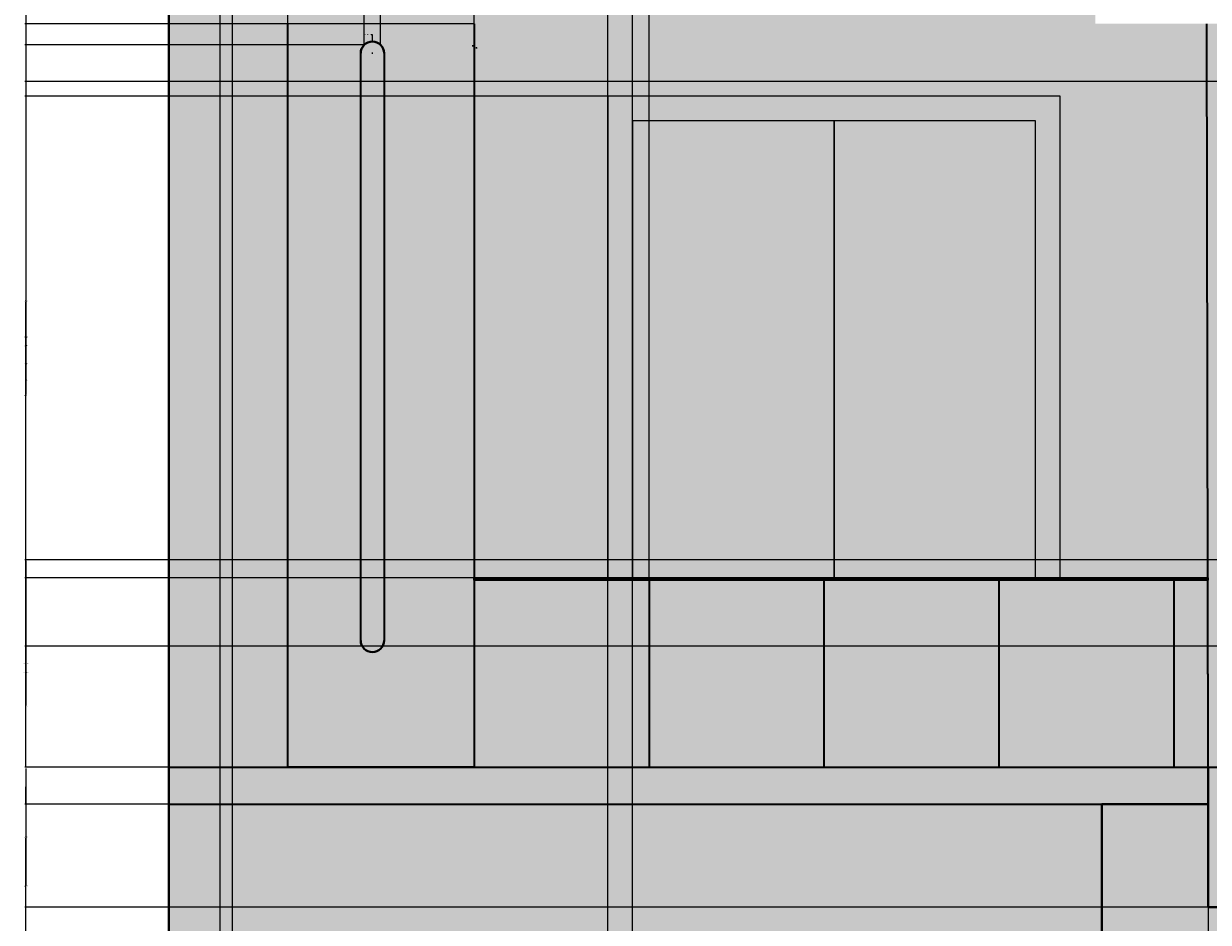
# Model space of a CAD drawing. Units: feet. Extents: x 2368 to 2738, y 1285 to 1782.
# Tile 2 of 6: x 2368 to 2561, y 1464 to 1610. Entities that reach past the tile are written whole.
import ezdxf

# ---------------------------------------------------------------- set-up
doc = ezdxf.new("R2010")
doc.units = ezdxf.units.FT
for name, color, linetype, lineweight in [('A-ANNO-DIMS', 2, 'Continuous', 18), ('A-DOOR', 3, 'Continuous', 25), ('A-ELEV', 7, 'Continuous', 35), ('A-ELEV-PATT', 252, 'Continuous', 13)]:
    doc.layers.add(name, color=color, linetype=linetype, lineweight=lineweight)
doc.styles.get("Standard").update_dxf_attribs({"font": 'arial.ttf'})
doc.dimstyles.get("Standard").update_dxf_attribs({"dimtxt": 0.18, "dimasz": 0.18, "dimexe": 0.18, "dimexo": 0.0625, "dimgap": 0.09, "dimtad": 0, "dimtih": 1, "dimtoh": 1, "dimdec": 1, "dimzin": 0, "dimdsep": 46, "dimlunit": 3, "dimtxsty": 'Standard', "dimcen": 0.09, "dimadec": 0, "dimazin": 0, "dimtfac": 1, "dimtdec": 1, "dimtofl": 0, "dimtmove": 0, "dimatfit": 3, "dimfxl": 1, "dimtolj": 1, "dimtzin": 0, "dimarcsym": 0})

# ---------------------------------------------------------------- blocks, each defined once
blk = doc.blocks.new('*D6')
at = {"layer": 'A-ANNO-DIMS', "color": 0, "lineweight": -2, "transparency": 16777216}
for p, q in [((2391.48, 1482.86), (2368.11, 1482.86)), ((2368.29, 1482.68), (2368.29, 1469.65)), ((2368.29, 1456.26), (2368.29, 1469.29)), ((2399.84, 1456.08), (2368.11, 1456.08))]:
    blk.add_line(p, q, dxfattribs=at)
at = {"layer": 'A-ANNO-DIMS', "color": 0, "transparency": 16777216}
for points in [[(2368.26, 1482.68), (2368.32, 1482.68), (2368.29, 1482.86)], [(2368.26, 1456.26), (2368.32, 1456.26), (2368.29, 1456.08)]]:
    blk.add_solid(points, dxfattribs=at)
at = {"layer": 'Defpoints', "color": 0, "transparency": 16777216}
for p in [(2368.29, 1482.86), (2391.54, 1482.86), (2399.91, 1456.08)]:
    blk.add_point(p, dxfattribs=at)
at = {"layer": 'A-ANNO-DIMS', "color": 0, "transparency": 16777216, "insert": (2368.29, 1469.47), "char_height": 0.18, "attachment_point": 5}
blk.add_mtext('\\A1;26.77', dxfattribs=at)
blk = doc.blocks.new('*D7')
at = {"layer": 'A-ANNO-DIMS', "color": 0, "lineweight": -2, "transparency": 16777216}
for p, q in [((2391.48, 1488.86), (2368.11, 1488.86)), ((2368.29, 1488.68), (2368.29, 1486.04)), ((2368.29, 1483.04), (2368.29, 1485.67)), ((2391.48, 1482.86), (2368.11, 1482.86))]:
    blk.add_line(p, q, dxfattribs=at)
at = {"layer": 'A-ANNO-DIMS', "color": 0, "transparency": 16777216}
for points in [[(2368.26, 1488.68), (2368.32, 1488.68), (2368.29, 1488.86)], [(2368.26, 1483.04), (2368.32, 1483.04), (2368.29, 1482.86)]]:
    blk.add_solid(points, dxfattribs=at)
at = {"layer": 'Defpoints', "color": 0, "transparency": 16777216}
for p in [(2368.29, 1488.86), (2391.54, 1488.86), (2391.54, 1482.86)]:
    blk.add_point(p, dxfattribs=at)
at = {"layer": 'A-ANNO-DIMS', "color": 0, "transparency": 16777216, "insert": (2368.29, 1485.86), "char_height": 0.18, "attachment_point": 5}
blk.add_mtext('\\A1;6', dxfattribs=at)
blk = doc.blocks.new('*D8')
at = {"layer": 'A-ANNO-DIMS', "color": 0, "lineweight": -2, "transparency": 16777216}
for p, q in [((2391.48, 1614.86), (2368.11, 1614.86)), ((2368.29, 1614.68), (2368.29, 1552.04)), ((2368.29, 1489.04), (2368.29, 1551.67)), ((2391.48, 1488.86), (2368.11, 1488.86))]:
    blk.add_line(p, q, dxfattribs=at)
at = {"layer": 'A-ANNO-DIMS', "color": 0, "transparency": 16777216}
for points in [[(2368.26, 1614.68), (2368.32, 1614.68), (2368.29, 1614.86)], [(2368.26, 1489.04), (2368.32, 1489.04), (2368.29, 1488.86)]]:
    blk.add_solid(points, dxfattribs=at)
at = {"layer": 'Defpoints', "color": 0, "transparency": 16777216}
for p in [(2368.29, 1614.86), (2391.54, 1614.86), (2391.54, 1488.86)]:
    blk.add_point(p, dxfattribs=at)
at = {"layer": 'A-ANNO-DIMS', "color": 0, "transparency": 16777216, "insert": (2368.29, 1551.86), "char_height": 0.18, "attachment_point": 5}
blk.add_mtext('\\A1;126', dxfattribs=at)
blk = doc.blocks.new('*D19')
at = {"layer": 'A-ANNO-DIMS', "color": 0, "lineweight": -2, "transparency": 16777216}
for p, q in [((2560.8, 1466.04), (2560.8, 1285.43)), ((2543.45, 1350.79), (2543.45, 1285.43)), ((2543.63, 1285.61), (2551.74, 1285.61)), ((2560.62, 1285.61), (2552.51, 1285.61))]:
    blk.add_line(p, q, dxfattribs=at)
at = {"layer": 'A-ANNO-DIMS', "color": 0, "transparency": 16777216}
for points in [[(2543.63, 1285.64), (2543.63, 1285.58), (2543.45, 1285.61)], [(2560.62, 1285.64), (2560.62, 1285.58), (2560.8, 1285.61)]]:
    blk.add_solid(points, dxfattribs=at)
at = {"layer": 'Defpoints', "color": 0, "transparency": 16777216}
for p in [(2560.8, 1466.1), (2543.45, 1350.86), (2560.8, 1285.61)]:
    blk.add_point(p, dxfattribs=at)
at = {"layer": 'A-ANNO-DIMS', "color": 0, "transparency": 16777216, "insert": (2552.12, 1285.61), "char_height": 0.18, "attachment_point": 5}
blk.add_mtext('\\A1;17.35', dxfattribs=at)
blk = doc.blocks.new('*D24')
at = {"layer": 'A-ANNO-DIMS', "color": 0, "lineweight": -2, "transparency": 16777216}
for p, q in [((2399.91, 1456.15), (2399.91, 1782.11)), ((2400.09, 1781.93), (2400.76, 1781.93)), ((2401.73, 1781.93), (2401.06, 1781.93)), ((2401.91, 1454.15), (2401.91, 1782.11))]:
    blk.add_line(p, q, dxfattribs=at)
at = {"layer": 'A-ANNO-DIMS', "color": 0, "transparency": 16777216}
for points in [[(2400.09, 1781.96), (2400.09, 1781.9), (2399.91, 1781.93)], [(2401.73, 1781.96), (2401.73, 1781.9), (2401.91, 1781.93)]]:
    blk.add_solid(points, dxfattribs=at)
at = {"layer": 'Defpoints', "color": 0, "transparency": 16777216}
for p in [(2401.91, 1781.93), (2399.91, 1456.08), (2401.91, 1454.08)]:
    blk.add_point(p, dxfattribs=at)
at = {"layer": 'A-ANNO-DIMS', "color": 0, "transparency": 16777216, "insert": (2400.91, 1781.93), "char_height": 0.18, "attachment_point": 5}
blk.add_mtext('\\A1;2', dxfattribs=at)
blk = doc.blocks.new('*D30')
at = {"layer": 'A-ANNO-DIMS', "color": 0, "lineweight": -2, "transparency": 16777216}
for p, q in [((2463.03, 1460.16), (2463.03, 1782.11)), ((2463.21, 1781.93), (2464.88, 1781.93)), ((2466.85, 1781.93), (2465.18, 1781.93)), ((2467.03, 1456.16), (2467.03, 1782.11))]:
    blk.add_line(p, q, dxfattribs=at)
at = {"layer": 'A-ANNO-DIMS', "color": 0, "transparency": 16777216}
for points in [[(2463.21, 1781.96), (2463.21, 1781.9), (2463.03, 1781.93)], [(2466.85, 1781.96), (2466.85, 1781.9), (2467.03, 1781.93)]]:
    blk.add_solid(points, dxfattribs=at)
at = {"layer": 'Defpoints', "color": 0, "transparency": 16777216}
for p in [(2467.03, 1781.93), (2463.03, 1460.1), (2467.03, 1456.1)]:
    blk.add_point(p, dxfattribs=at)
at = {"layer": 'A-ANNO-DIMS', "color": 0, "transparency": 16777216, "insert": (2465.03, 1781.93), "char_height": 0.18, "attachment_point": 5}
blk.add_mtext('\\A1;4', dxfattribs=at)
blk = doc.blocks.new('*D36')
at = {"layer": 'A-ANNO-DIMS', "color": 0, "lineweight": -2, "transparency": 16777216}
for p, q in [((2701.6, 1488.86), (2368.11, 1488.86)), ((2368.29, 1488.68), (2368.29, 1477.66)), ((2368.29, 1466.28), (2368.29, 1477.3)), ((2701.6, 1466.1), (2368.11, 1466.1))]:
    blk.add_line(p, q, dxfattribs=at)
at = {"layer": 'A-ANNO-DIMS', "color": 0, "transparency": 16777216}
for points in [[(2368.26, 1488.68), (2368.32, 1488.68), (2368.29, 1488.86)], [(2368.26, 1466.28), (2368.32, 1466.28), (2368.29, 1466.1)]]:
    blk.add_solid(points, dxfattribs=at)
at = {"layer": 'Defpoints', "color": 0, "transparency": 16777216}
for p in [(2368.29, 1488.86), (2701.66, 1488.86), (2701.66, 1466.1)]:
    blk.add_point(p, dxfattribs=at)
at = {"layer": 'A-ANNO-DIMS', "color": 0, "transparency": 16777216, "insert": (2368.29, 1477.48), "char_height": 0.18, "attachment_point": 5}
blk.add_mtext('\\A1;22.754', dxfattribs=at)
blk = doc.blocks.new('*D37')
at = {"layer": 'A-ANNO-DIMS', "color": 0, "lineweight": -2, "transparency": 16777216}
for p, q in [((2701.6, 1522.63), (2368.11, 1522.63)), ((2368.29, 1522.45), (2368.29, 1505.93)), ((2368.29, 1489.04), (2368.29, 1505.56)), ((2701.6, 1488.86), (2368.11, 1488.86))]:
    blk.add_line(p, q, dxfattribs=at)
at = {"layer": 'A-ANNO-DIMS', "color": 0, "transparency": 16777216}
for points in [[(2368.26, 1522.45), (2368.32, 1522.45), (2368.29, 1522.63)], [(2368.26, 1489.04), (2368.32, 1489.04), (2368.29, 1488.86)]]:
    blk.add_solid(points, dxfattribs=at)
at = {"layer": 'Defpoints', "color": 0, "transparency": 16777216}
for p in [(2368.29, 1522.63), (2701.66, 1522.63), (2701.66, 1488.86)]:
    blk.add_point(p, dxfattribs=at)
at = {"layer": 'A-ANNO-DIMS', "color": 0, "transparency": 16777216, "insert": (2368.29, 1505.74), "char_height": 0.18, "attachment_point": 5}
blk.add_mtext('\\A1;33.776', dxfattribs=at)
blk = doc.blocks.new('*D41')
at = {"layer": 'A-ANNO-DIMS', "color": 0, "lineweight": -2, "transparency": 16777216}
for p, q in [((2391.54, 1488.92), (2391.54, 1782.11)), ((2391.72, 1781.93), (2400.79, 1781.93)), ((2410.77, 1781.93), (2401.7, 1781.93)), ((2410.95, 1488.92), (2410.95, 1782.11))]:
    blk.add_line(p, q, dxfattribs=at)
at = {"layer": 'A-ANNO-DIMS', "color": 0, "transparency": 16777216}
for points in [[(2391.72, 1781.96), (2391.72, 1781.9), (2391.54, 1781.93)], [(2410.77, 1781.96), (2410.77, 1781.9), (2410.95, 1781.93)]]:
    blk.add_solid(points, dxfattribs=at)
at = {"layer": 'Defpoints', "color": 0, "transparency": 16777216}
for p in [(2410.95, 1781.93), (2391.54, 1488.86), (2410.95, 1488.86)]:
    blk.add_point(p, dxfattribs=at)
at = {"layer": 'A-ANNO-DIMS', "color": 0, "transparency": 16777216, "insert": (2401.24, 1781.93), "char_height": 0.18, "attachment_point": 5}
blk.add_mtext('\\A1;19.406', dxfattribs=at)
blk = doc.blocks.new('*D42')
at = {"layer": 'A-ANNO-DIMS', "color": 0, "lineweight": -2, "transparency": 16777216}
for p, q in [((2410.88, 1609.91), (2368.11, 1609.91)), ((2368.29, 1609.73), (2368.29, 1549.56)), ((2368.29, 1489.04), (2368.29, 1549.2)), ((2410.88, 1488.86), (2368.11, 1488.86))]:
    blk.add_line(p, q, dxfattribs=at)
at = {"layer": 'A-ANNO-DIMS', "color": 0, "transparency": 16777216}
for points in [[(2368.26, 1609.73), (2368.32, 1609.73), (2368.29, 1609.91)], [(2368.26, 1489.04), (2368.32, 1489.04), (2368.29, 1488.86)]]:
    blk.add_solid(points, dxfattribs=at)
at = {"layer": 'Defpoints', "color": 0, "transparency": 16777216}
for p in [(2368.29, 1609.91), (2410.95, 1609.91), (2410.95, 1488.86)]:
    blk.add_point(p, dxfattribs=at)
at = {"layer": 'A-ANNO-DIMS', "color": 0, "transparency": 16777216, "insert": (2368.29, 1549.38), "char_height": 0.18, "attachment_point": 5}
blk.add_mtext('\\A1;121.05', dxfattribs=at)
blk = doc.blocks.new('*D43')
at = {"layer": 'A-ANNO-DIMS', "color": 0, "lineweight": -2, "transparency": 16777216}
for p, q in [((2410.95, 1609.97), (2410.95, 1782.11)), ((2411.13, 1781.93), (2416.69, 1781.93)), ((2423.16, 1781.93), (2417.6, 1781.93)), ((2423.34, 1606.5), (2423.34, 1782.11))]:
    blk.add_line(p, q, dxfattribs=at)
at = {"layer": 'A-ANNO-DIMS', "color": 0, "transparency": 16777216}
for points in [[(2411.13, 1781.96), (2411.13, 1781.9), (2410.95, 1781.93)], [(2423.16, 1781.96), (2423.16, 1781.9), (2423.34, 1781.93)]]:
    blk.add_solid(points, dxfattribs=at)
at = {"layer": 'Defpoints', "color": 0, "transparency": 16777216}
for p in [(2423.34, 1781.93), (2410.95, 1609.91), (2423.34, 1606.44)]:
    blk.add_point(p, dxfattribs=at)
at = {"layer": 'A-ANNO-DIMS', "color": 0, "transparency": 16777216, "insert": (2417.15, 1781.93), "char_height": 0.18, "attachment_point": 5}
blk.add_mtext('\\A1;12.396', dxfattribs=at)
blk = doc.blocks.new('*D44')
at = {"layer": 'A-ANNO-DIMS', "color": 0, "lineweight": -2, "transparency": 16777216}
for p, q in [((2423.34, 1606.5), (2423.34, 1782.11)), ((2423.52, 1781.93), (2424.36, 1781.93)), ((2425.85, 1781.93), (2425.01, 1781.93)), ((2426.03, 1606.5), (2426.03, 1782.11))]:
    blk.add_line(p, q, dxfattribs=at)
at = {"layer": 'A-ANNO-DIMS', "color": 0, "transparency": 16777216}
for points in [[(2423.52, 1781.96), (2423.52, 1781.9), (2423.34, 1781.93)], [(2425.85, 1781.96), (2425.85, 1781.9), (2426.03, 1781.93)]]:
    blk.add_solid(points, dxfattribs=at)
at = {"layer": 'Defpoints', "color": 0, "transparency": 16777216}
for p in [(2426.03, 1781.93), (2423.34, 1606.44), (2426.03, 1606.44)]:
    blk.add_point(p, dxfattribs=at)
at = {"layer": 'A-ANNO-DIMS', "color": 0, "transparency": 16777216, "insert": (2424.69, 1781.93), "char_height": 0.18, "attachment_point": 5}
blk.add_mtext('\\A1;2.69', dxfattribs=at)
blk = doc.blocks.new('*D45')
at = {"layer": 'A-ANNO-DIMS', "color": 0, "lineweight": -2, "transparency": 16777216}
for p, q in [((2426.03, 1606.5), (2426.03, 1782.11)), ((2426.21, 1781.93), (2433.19, 1781.93)), ((2441.07, 1781.93), (2434.1, 1781.93)), ((2441.25, 1609.97), (2441.25, 1782.11))]:
    blk.add_line(p, q, dxfattribs=at)
at = {"layer": 'A-ANNO-DIMS', "color": 0, "transparency": 16777216}
for points in [[(2426.21, 1781.96), (2426.21, 1781.9), (2426.03, 1781.93)], [(2441.07, 1781.96), (2441.07, 1781.9), (2441.25, 1781.93)]]:
    blk.add_solid(points, dxfattribs=at)
at = {"layer": 'Defpoints', "color": 0, "transparency": 16777216}
for p in [(2441.25, 1781.93), (2441.25, 1609.91), (2426.03, 1606.44)]:
    blk.add_point(p, dxfattribs=at)
at = {"layer": 'A-ANNO-DIMS', "color": 0, "transparency": 16777216, "insert": (2433.64, 1781.93), "char_height": 0.18, "attachment_point": 5}
blk.add_mtext('\\A1;15.216', dxfattribs=at)
blk = doc.blocks.new('*D46')
at = {"layer": 'A-ANNO-DIMS', "color": 0, "lineweight": -2, "transparency": 16777216}
for p, q in [((2422.98, 1508.55), (2368.11, 1508.55)), ((2368.29, 1508.37), (2368.29, 1498.89)), ((2368.29, 1489.04), (2368.29, 1498.52)), ((2441.19, 1488.86), (2368.11, 1488.86))]:
    blk.add_line(p, q, dxfattribs=at)
at = {"layer": 'A-ANNO-DIMS', "color": 0, "transparency": 16777216}
for points in [[(2368.26, 1508.37), (2368.32, 1508.37), (2368.29, 1508.55)], [(2368.26, 1489.04), (2368.32, 1489.04), (2368.29, 1488.86)]]:
    blk.add_solid(points, dxfattribs=at)
at = {"layer": 'Defpoints', "color": 0, "transparency": 16777216}
for p in [(2368.29, 1508.55), (2423.04, 1508.55), (2441.25, 1488.86)]:
    blk.add_point(p, dxfattribs=at)
at = {"layer": 'A-ANNO-DIMS', "color": 0, "transparency": 16777216, "insert": (2368.29, 1498.7), "char_height": 0.18, "attachment_point": 5}
blk.add_mtext('\\A1;19.7', dxfattribs=at)
blk = doc.blocks.new('*D47')
at = {"layer": 'A-ANNO-DIMS', "color": 0, "lineweight": -2, "transparency": 16777216}
for p, q in [((2423.28, 1606.44), (2368.11, 1606.44)), ((2368.29, 1606.26), (2368.29, 1557.68)), ((2368.29, 1508.73), (2368.29, 1557.32)), ((2422.98, 1508.55), (2368.11, 1508.55))]:
    blk.add_line(p, q, dxfattribs=at)
at = {"layer": 'A-ANNO-DIMS', "color": 0, "transparency": 16777216}
for points in [[(2368.26, 1606.26), (2368.32, 1606.26), (2368.29, 1606.44)], [(2368.26, 1508.73), (2368.32, 1508.73), (2368.29, 1508.55)]]:
    blk.add_solid(points, dxfattribs=at)
at = {"layer": 'Defpoints', "color": 0, "transparency": 16777216}
for p in [(2368.29, 1606.44), (2423.34, 1606.44), (2423.04, 1508.55)]:
    blk.add_point(p, dxfattribs=at)
at = {"layer": 'A-ANNO-DIMS', "color": 0, "transparency": 16777216, "insert": (2368.29, 1557.5), "char_height": 0.18, "attachment_point": 5}
blk.add_mtext('\\A1;97.89', dxfattribs=at)
blk = doc.blocks.new('*D48')
at = {"layer": 'A-ANNO-DIMS', "color": 0, "lineweight": -2, "transparency": 16777216}
for p, q in [((2441.19, 1519.71), (2368.11, 1519.71)), ((2368.29, 1519.53), (2368.29, 1504.47)), ((2368.29, 1489.04), (2368.29, 1504.1)), ((2441.19, 1488.86), (2368.11, 1488.86))]:
    blk.add_line(p, q, dxfattribs=at)
at = {"layer": 'A-ANNO-DIMS', "color": 0, "transparency": 16777216}
for points in [[(2368.26, 1519.53), (2368.32, 1519.53), (2368.29, 1519.71)], [(2368.26, 1489.04), (2368.32, 1489.04), (2368.29, 1488.86)]]:
    blk.add_solid(points, dxfattribs=at)
at = {"layer": 'Defpoints', "color": 0, "transparency": 16777216}
for p in [(2368.29, 1519.71), (2441.25, 1519.71), (2441.25, 1488.86)]:
    blk.add_point(p, dxfattribs=at)
at = {"layer": 'A-ANNO-DIMS', "color": 0, "transparency": 16777216, "insert": (2368.29, 1504.28), "char_height": 0.18, "attachment_point": 5}
blk.add_mtext('\\A1;30.856', dxfattribs=at)
blk = doc.blocks.new('*D49')
at = {"layer": 'A-ANNO-DIMS', "color": 0, "lineweight": -2, "transparency": 16777216}
for p, q in [((2441.19, 1609.91), (2368.11, 1609.91)), ((2368.29, 1609.73), (2368.29, 1564.99)), ((2368.29, 1519.89), (2368.29, 1564.63)), ((2441.19, 1519.71), (2368.11, 1519.71))]:
    blk.add_line(p, q, dxfattribs=at)
at = {"layer": 'A-ANNO-DIMS', "color": 0, "transparency": 16777216}
for points in [[(2368.26, 1609.73), (2368.32, 1609.73), (2368.29, 1609.91)], [(2368.26, 1519.89), (2368.32, 1519.89), (2368.29, 1519.71)]]:
    blk.add_solid(points, dxfattribs=at)
at = {"layer": 'Defpoints', "color": 0, "transparency": 16777216}
for p in [(2368.29, 1609.91), (2441.25, 1609.91), (2441.25, 1519.71)]:
    blk.add_point(p, dxfattribs=at)
at = {"layer": 'A-ANNO-DIMS', "color": 0, "transparency": 16777216, "insert": (2368.29, 1564.81), "char_height": 0.18, "attachment_point": 5}
blk.add_mtext('\\A1;90.2', dxfattribs=at)
blk = doc.blocks.new('*D50')
at = {"layer": 'A-ANNO-DIMS', "color": 0, "lineweight": -2, "transparency": 16777216}
for p, q in [((2441.25, 1519.77), (2441.25, 1782.11)), ((2441.43, 1781.93), (2455.03, 1781.93)), ((2469.55, 1781.93), (2455.96, 1781.93)), ((2469.73, 1519.4), (2469.73, 1782.11))]:
    blk.add_line(p, q, dxfattribs=at)
at = {"layer": 'A-ANNO-DIMS', "color": 0, "transparency": 16777216}
for points in [[(2441.43, 1781.96), (2441.43, 1781.9), (2441.25, 1781.93)], [(2469.55, 1781.96), (2469.55, 1781.9), (2469.73, 1781.93)]]:
    blk.add_solid(points, dxfattribs=at)
at = {"layer": 'Defpoints', "color": 0, "transparency": 16777216}
for p in [(2469.73, 1781.93), (2441.25, 1519.71), (2469.73, 1519.33)]:
    blk.add_point(p, dxfattribs=at)
at = {"layer": 'A-ANNO-DIMS', "color": 0, "transparency": 16777216, "insert": (2455.49, 1781.93), "char_height": 0.18, "attachment_point": 5}
blk.add_mtext('\\A1;28.486', dxfattribs=at)
blk = doc.blocks.new('*D51')
at = {"layer": 'A-ANNO-DIMS', "color": 0, "lineweight": -2, "transparency": 16777216}
for p, q in [((2462.97, 1598.1), (2368.11, 1598.1)), ((2368.29, 1597.92), (2368.29, 1559.09)), ((2368.29, 1519.89), (2368.29, 1558.72)), ((2462.97, 1519.71), (2368.11, 1519.71))]:
    blk.add_line(p, q, dxfattribs=at)
at = {"layer": 'A-ANNO-DIMS', "color": 0, "transparency": 16777216}
for points in [[(2368.26, 1597.92), (2368.32, 1597.92), (2368.29, 1598.1)], [(2368.26, 1519.89), (2368.32, 1519.89), (2368.29, 1519.71)]]:
    blk.add_solid(points, dxfattribs=at)
at = {"layer": 'Defpoints', "color": 0, "transparency": 16777216}
for p in [(2368.29, 1598.1), (2463.03, 1598.1), (2463.03, 1519.71)]:
    blk.add_point(p, dxfattribs=at)
at = {"layer": 'A-ANNO-DIMS', "color": 0, "transparency": 16777216, "insert": (2368.29, 1558.9), "char_height": 0.18, "attachment_point": 5}
blk.add_mtext('\\A1;78.39', dxfattribs=at)
blk = doc.blocks.new('*D52')
at = {"layer": 'A-ANNO-DIMS', "color": 0, "lineweight": -2, "transparency": 16777216}
for p, q in [((2463.03, 1598.16), (2463.03, 1782.11)), ((2463.21, 1781.93), (2464.88, 1781.93)), ((2466.85, 1781.93), (2465.18, 1781.93)), ((2467.03, 1594.16), (2467.03, 1782.11))]:
    blk.add_line(p, q, dxfattribs=at)
at = {"layer": 'A-ANNO-DIMS', "color": 0, "transparency": 16777216}
for points in [[(2463.21, 1781.96), (2463.21, 1781.9), (2463.03, 1781.93)], [(2466.85, 1781.96), (2466.85, 1781.9), (2467.03, 1781.93)]]:
    blk.add_solid(points, dxfattribs=at)
at = {"layer": 'Defpoints', "color": 0, "transparency": 16777216}
for p in [(2467.03, 1781.93), (2463.03, 1598.1), (2467.03, 1594.1)]:
    blk.add_point(p, dxfattribs=at)
at = {"layer": 'A-ANNO-DIMS', "color": 0, "transparency": 16777216, "insert": (2465.03, 1781.93), "char_height": 0.18, "attachment_point": 5}
blk.add_mtext('\\A1;4', dxfattribs=at)
blk = doc.blocks.new('*D60')
at = {"layer": 'A-ANNO-DIMS', "color": 0, "lineweight": -2, "transparency": 16777216}
for p, q in [((2597.71, 1600.48), (2368.11, 1600.48)), ((2368.29, 1600.3), (2368.29, 1554.7)), ((2368.29, 1508.74), (2368.29, 1554.34)), ((2597.71, 1508.56), (2368.11, 1508.56))]:
    blk.add_line(p, q, dxfattribs=at)
at = {"layer": 'A-ANNO-DIMS', "color": 0, "transparency": 16777216}
for points in [[(2368.26, 1600.3), (2368.32, 1600.3), (2368.29, 1600.48)], [(2368.26, 1508.74), (2368.32, 1508.74), (2368.29, 1508.56)]]:
    blk.add_solid(points, dxfattribs=at)
at = {"layer": 'Defpoints', "color": 0, "transparency": 16777216}
for p in [(2368.29, 1600.48), (2597.78, 1600.48), (2597.78, 1508.56)]:
    blk.add_point(p, dxfattribs=at)
at = {"layer": 'A-ANNO-DIMS', "color": 0, "transparency": 16777216, "insert": (2368.29, 1554.52), "char_height": 0.18, "attachment_point": 5}
blk.add_mtext('\\A1;91.92', dxfattribs=at)
blk = doc.blocks.new('*D74')
at = {"layer": 'A-ANNO-DIMS', "color": 0, "lineweight": -2, "transparency": 16777216}
for p, q in [((2411.53, 1645.45), (2411.71, 1645.45)), ((2411.71, 1645.45), (2422.83, 1630.8)), ((2441.56, 1606), (2441.74, 1606)), ((2441.65, 1605.91), (2441.65, 1606.09))]:
    blk.add_line(p, q, dxfattribs=at)
at = {"layer": 'A-ANNO-DIMS', "color": 0, "transparency": 16777216}
blk.add_solid([(2422.85, 1630.81), (2422.8, 1630.78), (2422.94, 1630.65)], dxfattribs=at)
at = {"layer": 'Defpoints', "color": 0, "transparency": 16777216}
for p in [(2422.94, 1630.65), (2441.65, 1606)]:
    blk.add_point(p, dxfattribs=at)
at = {"layer": 'A-ANNO-DIMS', "color": 0, "transparency": 16777216, "insert": (2411.05, 1645.45), "char_height": 0.18, "attachment_point": 5}
blk.add_mtext('\\A1;R30.95', dxfattribs=at)
blk = doc.blocks.new('*D76')
at = {"layer": 'A-ANNO-DIMS', "color": 0, "lineweight": -2, "transparency": 16777216}
for p, q in [((2408.79, 1642.69), (2408.97, 1642.69)), ((2408.97, 1642.69), (2420.88, 1629.19)), ((2440.95, 1606.32), (2441.13, 1606.32)), ((2441.04, 1606.23), (2441.04, 1606.41))]:
    blk.add_line(p, q, dxfattribs=at)
at = {"layer": 'A-ANNO-DIMS', "color": 0, "transparency": 16777216}
blk.add_solid([(2420.9, 1629.21), (2420.85, 1629.17), (2421, 1629.05)], dxfattribs=at)
at = {"layer": 'Defpoints', "color": 0, "transparency": 16777216}
for p in [(2421, 1629.05), (2441.04, 1606.32)]:
    blk.add_point(p, dxfattribs=at)
at = {"layer": 'A-ANNO-DIMS', "color": 0, "transparency": 16777216, "insert": (2408.19, 1642.69), "char_height": 0.18, "attachment_point": 5}
blk.add_mtext('\\A1;2X R30.3', dxfattribs=at)
blk = doc.blocks.new('*D77')
at = {"layer": 'A-ANNO-DIMS', "color": 0, "lineweight": -2, "transparency": 16777216}
for p, q in [((2424.48, 1608.14), (2424.66, 1608.14)), ((2424.66, 1608.14), (2424.67, 1607.18)), ((2424.6, 1605.1), (2424.78, 1605.1)), ((2424.69, 1605.01), (2424.69, 1605.19))]:
    blk.add_line(p, q, dxfattribs=at)
at = {"layer": 'A-ANNO-DIMS', "color": 0, "transparency": 16777216}
blk.add_solid([(2424.7, 1607.18), (2424.64, 1607.18), (2424.67, 1607)], dxfattribs=at)
at = {"layer": 'Defpoints', "color": 0, "transparency": 16777216}
for p in [(2424.67, 1607), (2424.69, 1605.1)]:
    blk.add_point(p, dxfattribs=at)
at = {"layer": 'A-ANNO-DIMS', "color": 0, "transparency": 16777216, "insert": (2423.88, 1608.14), "char_height": 0.18, "attachment_point": 5}
blk.add_mtext('\\A1;2X R1.90', dxfattribs=at)

msp = doc.modelspace()

# ---------------------------------------------------------------- hatches: boundary and pattern name
at = {"layer": 'A-ELEV-PATT'}
h = msp.add_hatch(color=256, dxfattribs=at)
h.set_gradient(color1=(192, 192, 192), color2=(192, 192, 192), tint=1)
h.paths.add_polyline_path([(2714.1625, 1758.6751), (2519.621, 1758.6751), (2519.621, 1716.8552), (2714.1625, 1716.8552)])
h.paths.add_polyline_path([(2701.6591, 1693.9847), (2714.1625, 1693.9847), (2714.1625, 1710.8552), (2519.621, 1710.8552), (2519.621, 1662.8552), (2592.4132, 1662.8552), (2592.4132, 1689.493), (2665.1962, 1689.493), (2665.1962, 1662.8552), (2701.6591, 1662.8552)])
h.paths.add_polyline_path([(2701.6591, 1609.9058), (2597.776, 1609.9058), (2597.776, 1600.4784), (2665.1962, 1600.4784), (2665.1962, 1596.3371), (2665.1962, 1522.6314), (2701.6591, 1522.6314)])
h.paths.add_polyline_path([(2463.0324, 1598.097), (2536.677, 1598.097), (2536.677, 1519.7115), (2560.74, 1519.7115), (2560.5754, 1609.9058), (2542.3749, 1609.9058), (2441.2488, 1609.9058), (2441.2488, 1519.7115), (2463.0324, 1519.7115)])
h.paths.add_polyline_path([(2506.1956, 1662.8552), (2391.5414, 1662.8552), (2391.5414, 1644.4206), (2438.815, 1644.4206, -0.34592239), (2445.9507, 1638.8128), (2506.1956, 1638.8128)])
h.paths.add_polyline_path([(2410.9473, 1609.9058, -0.04175491), (2411.9608, 1614.8552), (2391.5414, 1614.8552), (2391.5414, 1488.8552), (2410.9473, 1488.8552)])
h.paths.add_polyline_path([(2426.5897, 1605.0962, 1), (2422.7862, 1605.0962), (2422.7862, 1509.5049, 1), (2426.5897, 1509.5049)])
h.paths.add_polyline_path([(2463.0324, 1460.097), (2536.677, 1460.097), (2536.677, 1350.8552), (2543.4468, 1350.8552), (2543.4468, 1482.8552), (2391.5414, 1482.8552), (2391.5414, 1350.8552), (2463.0324, 1350.8552)])
h.paths.add_polyline_path([(2436.8485, 1456.084), (2436.8485, 1379.669), (2399.9065, 1379.669), (2399.9065, 1456.084)], flags=16)
h.paths.add_polyline_path([(2434.8485, 1454.084), (2434.8485, 1381.669), (2401.9065, 1381.669), (2401.9065, 1454.084)], flags=0)
h.paths.add_polyline_path([(2714.1625, 1350.8552), (2391.5414, 1350.8552), (2391.5414, 1320.8552), (2714.1625, 1320.8552)])
h.paths.add_polyline_path([(2714.1625, 1320.8552), (2391.5414, 1320.8552), (2391.5414, 1308.8552), (2714.1625, 1308.8552)])
h = msp.add_hatch(color=256, dxfattribs=at)
h.set_gradient(color1=(255, 255, 255), tint=1)
h.paths.add_polyline_path([(2595.4132, 1686.493), (2662.1962, 1686.493), (2662.1962, 1662.8552), (2665.1962, 1662.8552), (2665.1962, 1689.493), (2592.4132, 1689.493), (2592.4132, 1662.8552), (2595.4132, 1662.8552)])
h.paths.add_polyline_path([(2665.1962, 1600.4784), (2597.776, 1600.4784), (2597.776, 1597.4784), (2662.1962, 1597.4784), (2662.1962, 1510.3225), (2597.776, 1510.3225), (2597.776, 1507.3225), (2665.1962, 1507.3225)])
h.paths.add_polyline_path([(2665.1962, 1461.1396), (2592.4132, 1461.1396), (2592.4132, 1367.9838), (2665.1962, 1367.9838)])
h.paths.add_polyline_path([(2662.1962, 1458.1396), (2662.1962, 1370.9838), (2595.4132, 1370.9838), (2595.4132, 1458.1396)], flags=16)
h.paths.add_polyline_path([(2593.776, 1609.9058), (2584.2358, 1609.9058), (2584.2358, 1488.8552), (2593.776, 1488.8552)])
h.paths.add_polyline_path([(2597.776, 1609.9058), (2595.4517, 1609.9058), (2595.4517, 1488.8552), (2597.776, 1488.8552)])
h.paths.add_polyline_path([(2569.8357, 1609.9058), (2560.5754, 1609.9058), (2560.74, 1519.7115), (2560.7407, 1519.7115), (2560.7407, 1519.3328), (2560.7963, 1488.8552), (2569.8357, 1488.8552)])
h.paths.add_polyline_path([(2572.6807, 1609.9058), (2571.6967, 1609.9058), (2571.6967, 1488.8552), (2572.6807, 1488.8552)])
h.paths.add_polyline_path([(2575.8428, 1609.9058), (2574.5416, 1609.9058), (2574.5416, 1488.8552), (2575.8428, 1488.8552)])
h.paths.add_polyline_path([(2579.0308, 1609.9058), (2577.7037, 1609.9058), (2577.7037, 1488.8552), (2579.0308, 1488.8552)])
h.paths.add_polyline_path([(2582.3749, 1609.9058), (2580.8918, 1609.9058), (2580.8918, 1488.8552), (2582.3749, 1488.8552)])
h = msp.add_hatch(color=256, dxfattribs=at)
h.set_gradient(color1=(242, 242, 242), color2=(242, 242, 242), tint=1)
h.paths.add_polyline_path([(2542.3749, 1636.6235), (2440.8236, 1636.6235, 0.37790365), (2410.9473, 1609.9058), (2410.9473, 1488.8552), (2441.2488, 1488.8552), (2441.2488, 1609.9058), (2542.3749, 1609.9058)])
h.paths.add_polyline_path([(2426.5897, 1605.0962), (2426.5897, 1509.5049, -1), (2422.7862, 1509.5049), (2422.7862, 1605.0962, -1)], flags=16)
h.paths.add_polyline_path([(2441.2488, 1636.6235), (2446.1448, 1636.6235, 0.43242195), (2438.815, 1644.4206), (2391.5414, 1644.4206), (2391.5414, 1620.8552), (2391.5414, 1614.8552), (2411.9608, 1614.8552, -0.33482359)])
h.paths.add_polyline_path([(2592.4132, 1461.1396), (2635.4878, 1461.1396), (2635.4878, 1466.101), (2560.7963, 1466.101), (2560.7963, 1482.8552), (2543.4468, 1482.8552), (2543.4468, 1350.8552), (2635.4878, 1350.8552), (2635.4878, 1367.9838), (2592.4132, 1367.9838)])
h = msp.add_hatch(color=256, dxfattribs=at)
h.set_gradient(color2=(0, 0, 0), tint=1)
h.paths.add_polyline_path([(2467.0324, 1594.097), (2532.677, 1594.097), (2532.677, 1519.7115), (2536.677, 1519.7115), (2536.677, 1598.097), (2463.0324, 1598.097), (2463.0324, 1519.7115), (2467.0324, 1519.7115)])
h.paths.add_polyline_path([(2536.677, 1460.097), (2463.0324, 1460.097), (2463.0324, 1350.8552), (2467.0324, 1350.8552), (2467.0324, 1456.097), (2532.677, 1456.097), (2532.677, 1350.8552), (2536.677, 1350.8552)])
h.paths.add_polyline_path([(2436.8485, 1456.084), (2399.9065, 1456.084), (2399.9065, 1379.669), (2436.8485, 1379.669)])
h.paths.add_polyline_path([(2401.9065, 1454.084), (2434.8485, 1454.084), (2434.8485, 1381.669), (2401.9065, 1381.669)], flags=16)
h = msp.add_hatch(color=256, dxfattribs=at)
h.set_gradient(color1=(89, 52, 3), color2=(89, 52, 3), tint=1)
h.paths.add_polyline_path([(2532.677, 1456.097), (2499.8547, 1456.097), (2499.8547, 1350.8552), (2532.677, 1350.8552)])
h.paths.add_polyline_path([(2499.8547, 1456.097), (2467.0324, 1456.097), (2467.0324, 1350.8552), (2499.8547, 1350.8552)])
h.paths.add_polyline_path([(2499.8547, 1594.097), (2467.0324, 1594.097), (2467.0324, 1519.7115), (2499.8547, 1519.7115)])
h.paths.add_polyline_path([(2532.677, 1594.097), (2499.8547, 1594.097), (2499.8547, 1519.7115), (2532.677, 1519.7115)])
h = msp.add_hatch(color=256, dxfattribs=at)
h.set_gradient(color1=(128, 128, 128), color2=(128, 128, 128), tint=1)
h.paths.add_polyline_path([(2560.7407, 1519.7115), (2441.2488, 1519.7115), (2441.2488, 1519.3328), (2560.7407, 1519.3328)])
h = msp.add_hatch(color=256, dxfattribs=at)
h.set_gradient(color1=(153, 185, 219), color2=(153, 185, 219), tint=1)
h.paths.add_polyline_path([(2469.7346, 1519.3328), (2441.2488, 1519.3328), (2441.2488, 1488.8552), (2469.7346, 1488.8552)])
h.paths.add_polyline_path([(2498.2204, 1519.3328), (2469.7346, 1519.3328), (2469.7346, 1488.8552), (2498.2204, 1488.8552)])
h.paths.add_polyline_path([(2526.7062, 1519.3328), (2499.8547, 1519.3328), (2499.8547, 1488.8552), (2526.7062, 1488.8552)])
h.paths.add_polyline_path([(2499.8547, 1519.3328), (2498.2204, 1519.3328), (2498.2204, 1488.8552), (2499.8547, 1488.8552)])
h = msp.add_hatch(color=256, dxfattribs=at)
h.set_gradient(color1=(153, 185, 219), color2=(153, 185, 219), tint=1)
h.paths.add_polyline_path([(2555.192, 1519.3328), (2526.7062, 1519.3328), (2526.7062, 1488.8552), (2555.192, 1488.8552)])
h.paths.add_polyline_path([(2560.7407, 1519.3328), (2555.192, 1519.3328), (2555.192, 1488.8552), (2560.7963, 1488.8552)])
h = msp.add_hatch(color=256, dxfattribs=at)
h.set_gradient(color1=(127, 31, 0), color2=(127, 31, 0), tint=1)
h.paths.add_polyline_path([(2560.7963, 1488.8552), (2391.5414, 1488.8552), (2391.5414, 1482.8552), (2560.7963, 1482.8552)])
h = msp.add_hatch(color=256, dxfattribs=at)
h.set_gradient(color1=(128, 128, 128), color2=(128, 128, 128), tint=1)
h.paths.add_polyline_path([(2701.6591, 1488.8552), (2560.7963, 1488.8552), (2560.7963, 1466.101), (2701.6591, 1466.101)])

# ---------------------------------------------------------------- linework, layer by layer
at = {"layer": 'A-DOOR'}
msp.add_line((2499.8547, 1594.097), (2499.8547, 1519.7115), dxfattribs=at)
for points in [[(2536.677, 1519.3328), (2536.677, 1598.097), (2463.0324, 1598.097), (2463.0324, 1519.7115)], [(2532.677, 1519.7115), (2532.677, 1594.097), (2467.0324, 1594.097), (2467.0324, 1519.7115)]]:
    msp.add_lwpolyline(points, dxfattribs=at)
msp.add_lwpolyline([(2499.8547, 1594.097), (2499.883, 1594.097), (2499.883, 1519.7115), (2499.8547, 1519.7115)], close=True, dxfattribs=at)
at = {"layer": 'A-ELEV'}
for p, q in [((2391.5414, 1644.4206), (2391.5414, 1308.8552)), ((2391.5414, 1488.8552), (2391.5414, 1614.8552)), ((2410.9473, 1488.8552), (2410.9473, 1609.9058)), ((2441.2488, 1609.9058), (2441.2488, 1488.8552)), ((2560.7963, 1488.8552), (2560.5754, 1609.9058)), ((2422.7862, 1509.5049), (2422.7862, 1605.0962)), ((2426.5897, 1605.0962), (2426.5897, 1509.5049)), ((2560.7407, 1519.3328), (2441.2488, 1519.7115)), ((2469.7346, 1519.3328), (2469.7346, 1488.8552)), ((2469.7346, 1519.3328), (2469.7346, 1488.8552)), ((2498.2204, 1519.3328), (2498.2204, 1488.8552)), ((2498.2204, 1519.3328), (2498.2204, 1488.8552)), ((2526.7062, 1519.3328), (2526.7062, 1488.9072)), ((2526.7062, 1519.3328), (2526.7062, 1488.9072)), ((2555.192, 1519.3328), (2555.192, 1488.8552)), ((2555.192, 1519.3328), (2555.192, 1488.8552)), ((2560.7963, 1488.8552), (2560.7407, 1519.3328)), ((2391.5414, 1482.8552), (2391.5414, 1488.8552)), ((2391.5414, 1488.8552), (2701.6591, 1488.8552)), ((2391.5414, 1488.8552), (2701.6591, 1488.8552)), ((2441.2488, 1488.8552), (2560.7963, 1488.8552)), ((2560.7963, 1466.101), (2560.7963, 1488.8552)), ((2560.7963, 1488.8552), (2701.6591, 1488.8552)), ((2560.7963, 1482.8552), (2560.7963, 1488.8552)), ((2560.7963, 1488.8552), (2560.7963, 1466.101)), ((2391.5414, 1350.8552), (2391.5414, 1482.8552)), ((2391.5414, 1482.8552), (2560.7963, 1482.8552)), ((2391.5414, 1482.8552), (2560.7963, 1482.8552)), ((2543.4468, 1350.8552), (2543.4468, 1482.8552)), ((2560.7963, 1482.8552), (2543.4468, 1482.8552)), ((2543.4468, 1482.8552), (2543.4468, 1350.8552)), ((2701.6591, 1466.101), (2560.7963, 1466.101)), ((2560.7963, 1466.101), (2701.6591, 1466.101))]:
    msp.add_line(p, q, dxfattribs=at)
msp.add_lwpolyline([(2441.2488, 1609.9058), (2441.2488, 1488.8552), (2410.9473, 1488.8552), (2410.9473, 1609.9058)], dxfattribs=at)
msp.add_lwpolyline([(2422.7862, 1509.5049), (2422.7862, 1605.0962, -1), (2426.5897, 1605.0962), (2426.5897, 1509.5049, -1)], format="xyb", close=True, dxfattribs=at)
msp.add_lwpolyline([(2441.2488, 1519.7115), (2560.7407, 1519.7115), (2560.7407, 1519.3328), (2441.2488, 1519.3328)], close=True, dxfattribs=at)
for centre, start, end in [((2424.6879, 1605.0962), 360, 180), ((2424.6879, 1509.5049), 180, 0)]:
    msp.add_arc(centre, 1.9018, start, end, dxfattribs=at)

# ---------------------------------------------------------------- dimensions: what is measured, and where the dimension line sits
at = {"layer": 'A-ANNO-DIMS'}
for base, p1, p2, override, picture, middle in [((2410.9473, 1781.9251), (2391.5414, 1488.8552), (2410.9473, 1488.8552), {"dimdec": 3, "dimlfac": 1, "dimrnd": 0, "dimzin": 0, "dimdsep": 46, "dimlunit": 2}, '*D41', (2401.2443, 1781.9251)), ((2401.9065, 1781.9251), (2399.9065, 1456.084), (2401.9065, 1454.084), {"dimdec": 0, "dimlfac": 1, "dimrnd": 0, "dimzin": 0, "dimdsep": 46, "dimlunit": 2}, '*D24', (2400.9065, 1781.9251)), ((2423.3432, 1781.9251), (2410.9473, 1609.9058), (2423.3432, 1606.4409), {"dimdec": 3, "dimlfac": 1, "dimrnd": 0, "dimzin": 0, "dimdsep": 46, "dimlunit": 2}, '*D43', (2417.1452, 1781.9251)), ((2426.0327, 1781.9251), (2423.3432, 1606.4409), (2426.0327, 1606.4409), {"dimdec": 2, "dimlfac": 1, "dimrnd": 0, "dimzin": 0, "dimdsep": 46, "dimlunit": 2}, '*D44', (2424.6879, 1781.9251)), ((2441.2488, 1781.9251), (2426.0327, 1606.4409), (2441.2488, 1609.9058), {"dimdec": 3, "dimlfac": 1, "dimrnd": 0, "dimzin": 0, "dimdsep": 46, "dimlunit": 2}, '*D45', (2433.6407, 1781.9251)), ((2469.7346, 1781.9251), (2441.2488, 1519.7115), (2469.7346, 1519.3328), {"dimdec": 3, "dimlfac": 1, "dimrnd": 0, "dimzin": 0, "dimdsep": 46, "dimlunit": 2}, '*D50', (2455.4917, 1781.9251)), ((2467.0324, 1781.9251), (2463.0324, 1460.097), (2467.0324, 1456.097), {"dimdec": 0, "dimlfac": 1, "dimrnd": 0, "dimzin": 0, "dimdsep": 46, "dimlunit": 2}, '*D30', (2465.0324, 1781.9251)), ((2467.0324, 1781.9251), (2463.0324, 1598.097), (2467.0324, 1594.097), {"dimdec": 0, "dimlfac": 1, "dimrnd": 0, "dimzin": 0, "dimdsep": 46, "dimlunit": 2}, '*D52', (2465.0324, 1781.9251)), ((2560.7963, 1285.6052), (2543.4468, 1350.8552), (2560.7963, 1466.101), {"dimdec": 2, "dimlfac": 1, "dimrnd": 0, "dimzin": 0, "dimdsep": 46, "dimlunit": 2}, '*D19', (2552.1216, 1285.6052))]:
    dim = msp.add_linear_dim(base=base, p1=p1, p2=p2, dimstyle='Standard', override=override, dxfattribs=at)
    dim.commit()
    dim.dimension.update_dxf_attribs({"geometry": picture, "text_midpoint": middle})
dim = msp.add_radius_dim(center=(2441.6514, 1605.9998), mpoint=(2422.9377, 1630.6534), dimstyle='Standard', override={"dimdec": 2, "dimlfac": 1, "dimrnd": 0, "dimzin": 0, "dimdsep": 46, "dimlunit": 2}, dxfattribs=at)
dim.commit()
dim.dimension.update_dxf_attribs({"geometry": '*D74', "text_midpoint": (2411.049, 1645.4455), "dimtype": 164})
for center, mpoint, override, picture, middle in [((2441.0362, 1606.3227), (2420.996, 1629.051), {"dimdec": 1, "dimlfac": 1, "dimrnd": 0, "dimzin": 0, "dimdsep": 46, "dimlunit": 2}, '*D76', (2408.1871, 1642.6879)), ((2424.6879, 1605.0962), (2424.6708, 1606.9978), {"dimdec": 2, "dimlfac": 1, "dimrnd": 0, "dimzin": 0, "dimdsep": 46, "dimlunit": 2}, '*D77', (2423.876, 1608.1389))]:
    dim = msp.add_radius_dim(center=center, mpoint=mpoint, text='2X <>', dimstyle='Standard', override=override, dxfattribs=at)
    dim.commit()
    dim.dimension.update_dxf_attribs({"geometry": picture, "text_midpoint": middle, "dimtype": 164})
for base, p1, p2, override, picture, middle in [((2368.2914, 1614.8552), (2391.5414, 1488.8552), (2391.5414, 1614.8552), {"dimdec": 0, "dimlfac": 1, "dimrnd": 0, "dimzin": 0, "dimdsep": 46, "dimlunit": 2}, '*D8', (2368.2914, 1551.8552)), ((2368.2914, 1609.9058), (2410.9473, 1488.8552), (2410.9473, 1609.9058), {"dimdec": 2, "dimlfac": 1, "dimrnd": 0, "dimzin": 0, "dimdsep": 46, "dimlunit": 2}, '*D42', (2368.2914, 1549.3805)), ((2368.2914, 1609.9058), (2441.2488, 1519.7115), (2441.2488, 1609.9058), {"dimdec": 1, "dimlfac": 1, "dimrnd": 0, "dimzin": 0, "dimdsep": 46, "dimlunit": 2}, '*D49', (2368.2914, 1564.8086)), ((2368.2914, 1606.4409), (2423.041, 1508.5541), (2423.3432, 1606.4409), {"dimdec": 2, "dimlfac": 1, "dimrnd": 0, "dimzin": 0, "dimdsep": 46, "dimlunit": 2}, '*D47', (2368.2914, 1557.4975)), ((2368.2914, 1600.4784), (2597.776, 1508.5593), (2597.776, 1600.4784), {"dimdec": 2, "dimlfac": 1, "dimrnd": 0, "dimzin": 0, "dimdsep": 46, "dimlunit": 2}, '*D60', (2368.2914, 1554.5188)), ((2368.2914, 1598.097), (2463.0324, 1519.7115), (2463.0324, 1598.097), {"dimdec": 2, "dimlfac": 1, "dimrnd": 0, "dimzin": 0, "dimdsep": 46, "dimlunit": 2}, '*D51', (2368.2914, 1558.9043)), ((2368.2914, 1522.6314), (2701.6591, 1488.8552), (2701.6591, 1522.6314), {"dimdec": 3, "dimlfac": 1, "dimrnd": 0, "dimzin": 0, "dimdsep": 46, "dimlunit": 2}, '*D37', (2368.2914, 1505.7433)), ((2368.2914, 1519.7115), (2441.2488, 1488.8552), (2441.2488, 1519.7115), {"dimdec": 3, "dimlfac": 1, "dimrnd": 0, "dimzin": 0, "dimdsep": 46, "dimlunit": 2}, '*D48', (2368.2914, 1504.2834)), ((2368.2914, 1508.5541), (2441.2488, 1488.8552), (2423.041, 1508.5541), {"dimdec": 1, "dimlfac": 1, "dimrnd": 0, "dimzin": 0, "dimdsep": 46, "dimlunit": 2}, '*D46', (2368.2914, 1498.7046)), ((2368.2914, 1488.8552), (2701.6591, 1466.101), (2701.6591, 1488.8552), {"dimdec": 3, "dimlfac": 1, "dimrnd": 0, "dimzin": 0, "dimdsep": 46, "dimlunit": 2}, '*D36', (2368.2914, 1477.4781)), ((2368.2914, 1488.8552), (2391.5414, 1482.8552), (2391.5414, 1488.8552), {"dimdec": 0, "dimlfac": 1, "dimrnd": 0, "dimzin": 0, "dimdsep": 46, "dimlunit": 2}, '*D7', (2368.2914, 1485.8552)), ((2368.2914, 1482.8552), (2399.9065, 1456.084), (2391.5414, 1482.8552), {"dimdec": 2, "dimlfac": 1, "dimrnd": 0, "dimzin": 0, "dimdsep": 46, "dimlunit": 2}, '*D6', (2368.2914, 1469.4696))]:
    dim = msp.add_linear_dim(base=base, p1=p1, p2=p2, angle=90, dimstyle='Standard', override=override, dxfattribs=at)
    dim.commit()
    dim.dimension.update_dxf_attribs({"geometry": picture, "text_midpoint": middle})

doc.saveas('drawing.dxf')
